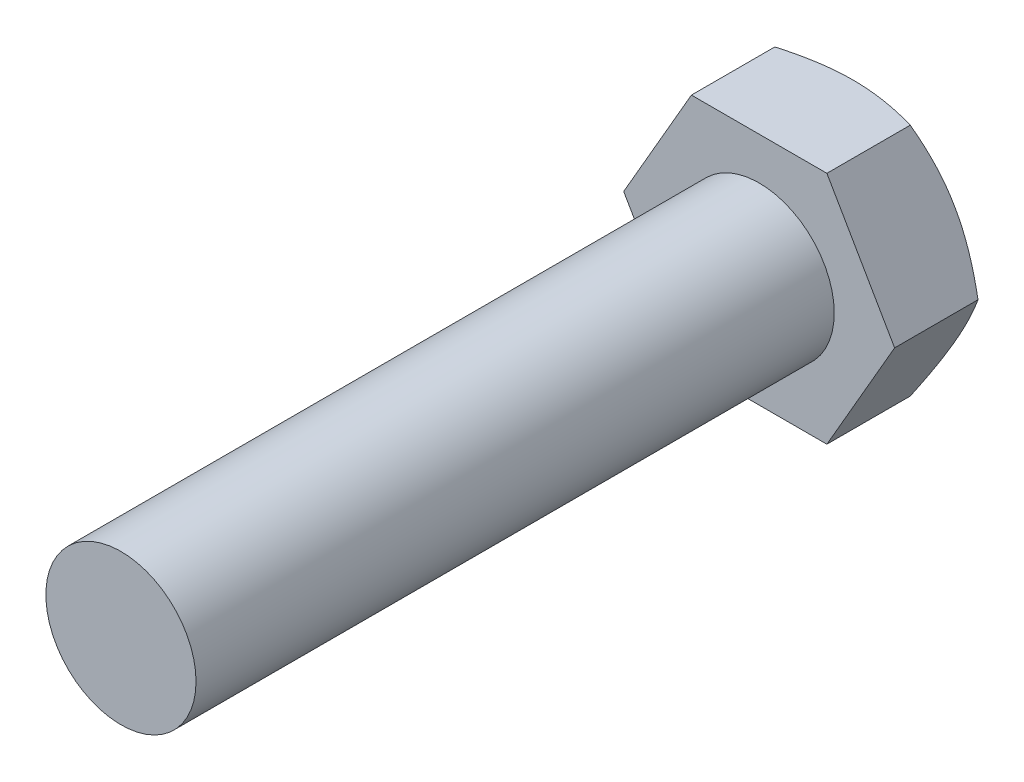
SolidWorks part; units mm, degrees
material "Plain Carbon Steel"
ref_plane "Front Plane" through (0, 0, 0) normal (0, 0, 1) x (1, 0, 0)
ref_plane "Top Plane" through (0, 0, 0) normal (0, 1, 0) x (1, 0, 0)
ref_plane "Right Plane" through (0, 0, 0) normal (1, 0, 0) x (0, 0, -1)
sketch "Hex Head Profile 25AF" plane through (0, 0, 0) normal (0, 0, 1) x (1, 0, 0)
  line L0 (0, 48.6222) -> (0, -44.0964) construction
  line L1 (-84.5231, 0) -> (84.7677, 0) construction
  line L3 (14.4338, 0) -> (7.2169, 12.5)
  line L4 (7.2169, 12.5) -> (-7.2169, 12.5)
  line L5 (-7.2169, 12.5) -> (-14.4338, 0)
  line L6 (-14.4338, 0) -> (-7.2169, -12.5)
  line L7 (-7.2169, -12.5) -> (7.2169, -12.5)
  line L8 (7.2169, -12.5) -> (14.4338, 0)
  circle A0 centre (0, 0) radius 12.5 construction
  dimension "D1" = 25
extrude "Hex Head 25AF x10" add sketch "Hex Head Profile 25AF" along normal blind 10
sketch "Head Chamfer Profile" plane through (0, 0, 0) normal (0, 0, -1) x (-1, 0, 0)
  circle A0 centre (0, 0) radius 12.5
  dimension "D1" = 25
extrude "Head Chamfer Cut" cut sketch "Head Chamfer Profile" against normal blind 10 draft 60 flip side to cut contours A0
sketch "Shank Profile Ø16" plane through (0, 0, 10) normal (0, 0, 1) x (1, 0, 0)
  circle A0 centre (0, 0) radius 8
  dimension "D1" = 16
extrude "Shank Ø16 x68" add sketch "Shank Profile Ø16" along normal blind 68
